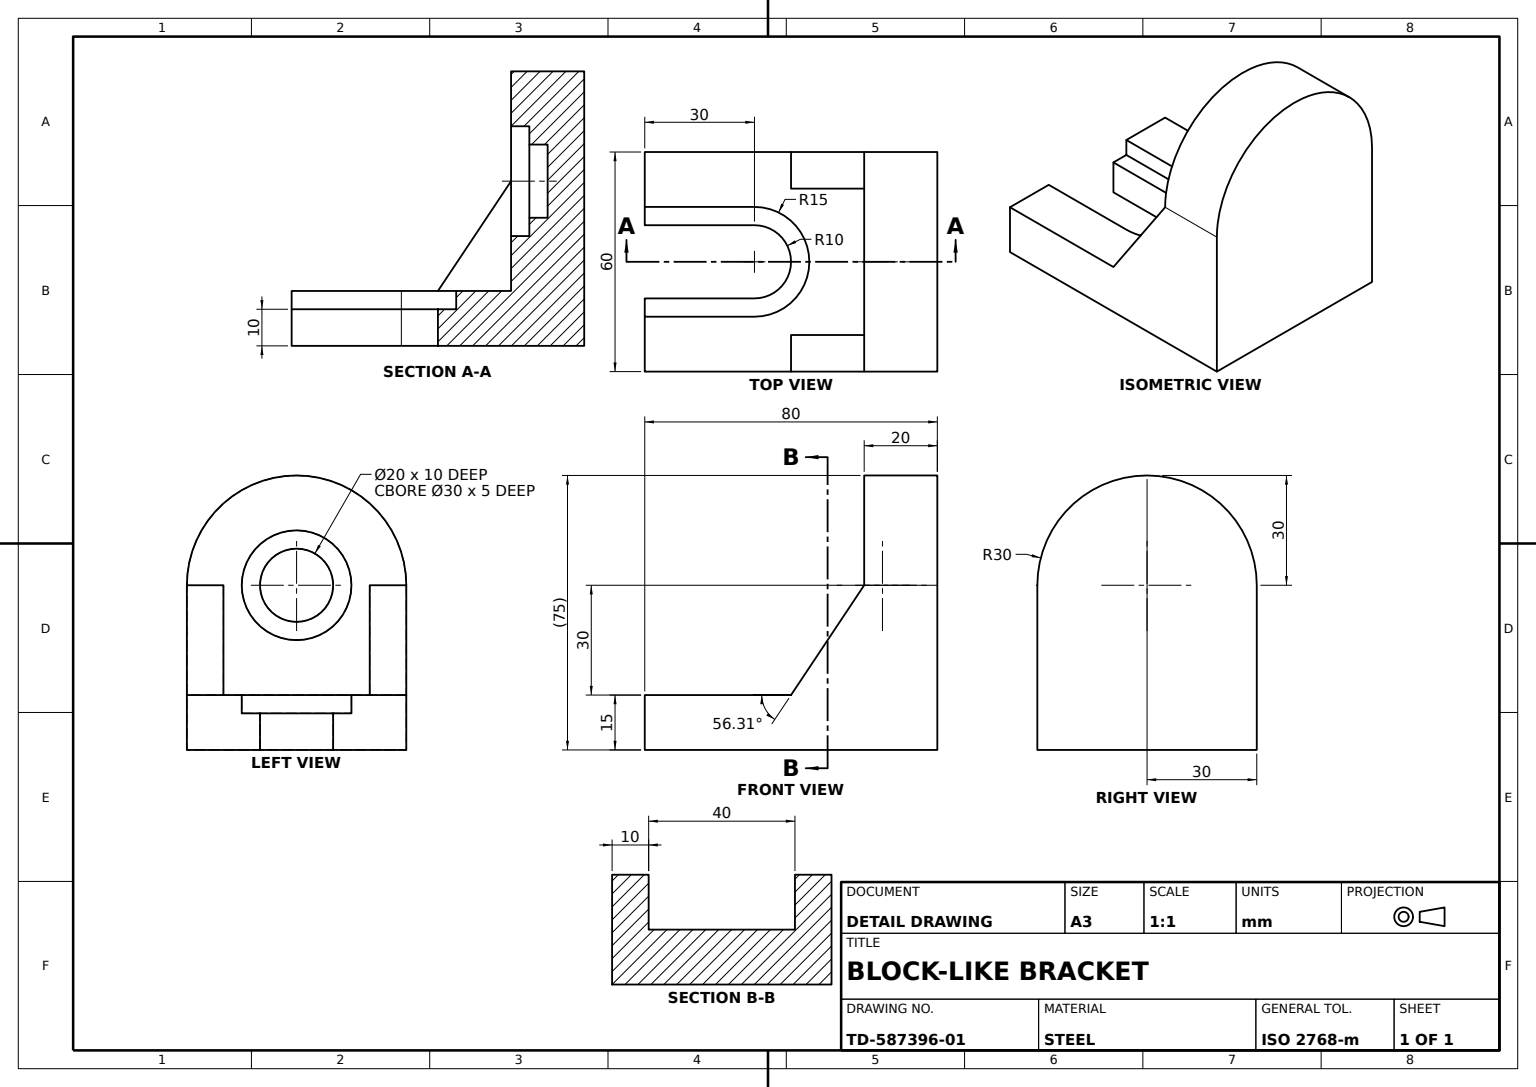
from build123d import *

# Parameters (mm, degrees)
BASE_PLATE_SKETCH_W = 80
BASE_PLATE_SKETCH_H = 60
BASE_PLATE_DEPTH    = 15
UPRIGHT_BLOCK_DEPTH = 20
RECESS_30_SKETCH_R  = 15
RECESS_30_DEPTH     = 5
RECESS_20_SKETCH_R  = 10
RECESS_20_DEPTH     = 5
SLOT_30_DEPTH       = 5
SLOT_STEP_20_DEPTH  = 10
SIDE_BOSS_DEPTH     = 10
ROUNDED_BOSS_DEPTH  = 10


with BuildPart() as part:
    # Base Plate Sketch → Base Plate (new body)
    with BuildSketch(Plane.XY):
        with Locations((40, 30)):
            Rectangle(BASE_PLATE_SKETCH_W, BASE_PLATE_SKETCH_H)
    extrude(amount=BASE_PLATE_DEPTH)

    # Upright Block Sketch → Upright Block (add)
    with BuildSketch(Plane(origin=(80, 0, 0), x_dir=(0, 0, -1), z_dir=(1, 0, 0))):
        with BuildLine():
            Line((-15, 60), (-45, 60))
            ThreePointArc((-45, 60), (-75, 30), (-45, 0))
            Line((-45, 0), (-15, 0))
            Line((-15, 0), (-15, 60))
        make_face()
    extrude(amount=-UPRIGHT_BLOCK_DEPTH)

    # Recess Ø30 Sketch → Recess Ø30 (cut)
    with BuildSketch(Plane.ZY.offset(-60)):
        with Locations((45, 30)):
            Circle(RECESS_30_SKETCH_R)
    extrude(amount=-RECESS_30_DEPTH, mode=Mode.SUBTRACT)

    # Recess Ø20 Sketch → Recess Ø20 (cut)
    with BuildSketch(Plane.ZY.offset(-65)):
        with Locations((45, 30)):
            Circle(RECESS_20_SKETCH_R)
    extrude(amount=-RECESS_20_DEPTH, mode=Mode.SUBTRACT)

    # Slot 30 Sketch → Slot 30 (cut)
    with BuildSketch(Plane.XY.offset(15)):
        with BuildLine():
            Line((0, 45), (0, 15))
            Line((0, 15), (30, 15))
            ThreePointArc((30, 15), (45, 30), (30, 45))
            Line((30, 45), (0, 45))
        make_face()
    extrude(amount=-SLOT_30_DEPTH, mode=Mode.SUBTRACT)

    # Slot Step 20 Sketch → Slot Step 20 (cut)
    with BuildSketch(Plane.XY.offset(10)):
        with BuildLine():
            Line((0, 40), (30, 40))
            ThreePointArc((30, 40), (40, 30), (30, 20))
            Line((30, 20), (0, 20))
            Line((0, 20), (0, 40))
        make_face()
    extrude(amount=-SLOT_STEP_20_DEPTH, mode=Mode.SUBTRACT)

    # Side Boss Sketch → Side Boss (add)
    with BuildSketch(Plane.XZ):
        Polygon((60, 45), (40, 15), (60, 15), align=None)
    extrude(amount=-SIDE_BOSS_DEPTH)

    # Rounded Boss Sketch → Rounded Boss (add)
    with BuildSketch(Plane(origin=(0, 60, 0), x_dir=(1, 0, 0), z_dir=(0, 1, 0))):
        Polygon((40, -15), (60, -15), (60, -45), align=None)
    extrude(amount=-ROUNDED_BOSS_DEPTH)


solid = part.part
